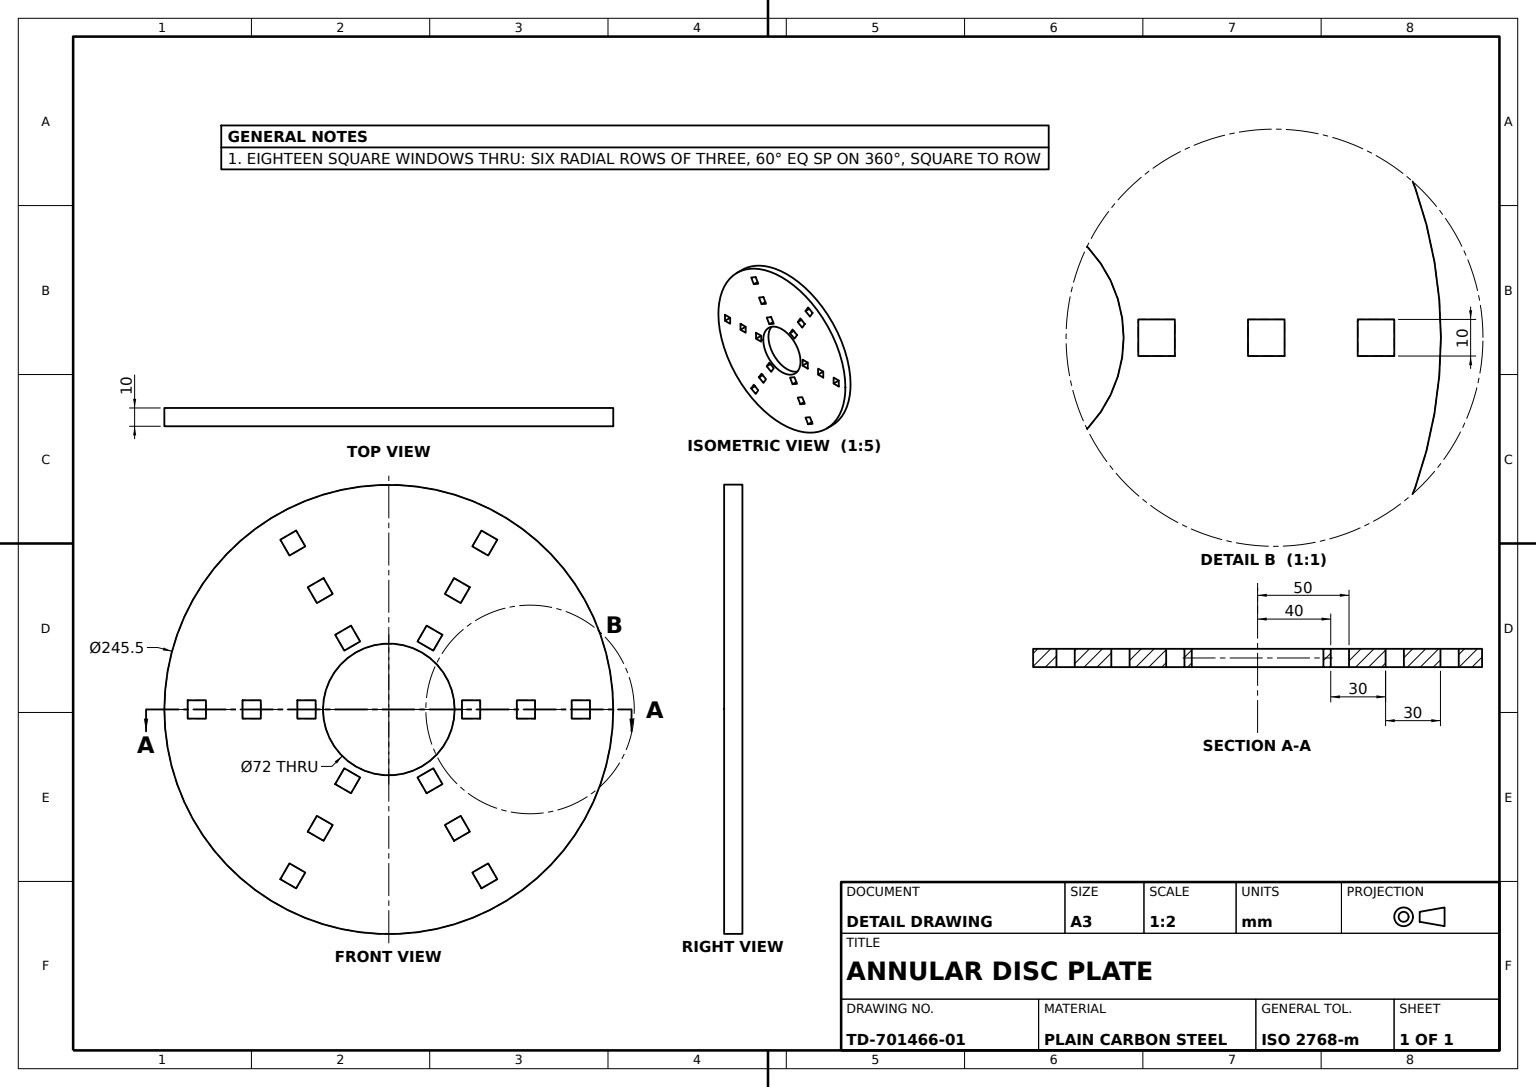
SolidWorks part; units mm, degrees
material "Plain Carbon Steel"
ref_plane "Front Plane" through (0, 0, 0) normal (0, 0, 1) x (1, 0, 0)
ref_plane "Top Plane" through (0, 0, 0) normal (0, 1, 0) x (1, 0, 0)
ref_plane "Right Plane" through (0, 0, 0) normal (1, 0, 0) x (0, 0, -1)
sketch "Plate Profile Ø245.5" plane through (0, 0, 0) normal (0, 0, 1) x (1, 0, 0)
  circle A0 centre (0, 0) radius 122.75
  dimension "D1" = 245.5
extrude "Plate Disc Ø245.5x10" add sketch "Plate Profile Ø245.5" along normal blind 10
sketch "Centre Bore Profile Ø72" plane through (0, 0, 10) normal (0, 0, 1) x (1, 0, 0)
  circle A0 centre (0, 0) radius 36
  dimension "D1" = 72
extrude "Centre Bore Ø72" cut sketch "Centre Bore Profile Ø72" against normal through all
sketch "Window Profile" plane through (0, 0, 10) normal (0, 0, 1) x (1, 0, 0)
  line L0 (0, 0) -> (0, 122.75) construction
  line L1 (0, 0) -> (0, -122.75) construction
  line L2 (0, 0) -> (40, 0)
  line L3 (0, 0) -> (-122.75, 0)
  line L4 (40, 0) -> (40, 5)
  line L5 (40, 0) -> (40, -5)
  line L6 (40, -5) -> (50, -5)
  line L7 (50, -5) -> (50, 5)
  line L8 (50, 5) -> (40, 5)
  line L9 (50, 0) -> (122.75, 0)
  circle A0 centre (0, 0) radius 122.75 construction
  circle A1 centre (0, 0) radius 36 construction
  dimension "D1" = 40
  dimension "D2" = 50
extrude "Window Cut" cut sketch "Window Profile" against normal through all contours L7 L8 L4 L5 L6
ref_plane "Plane1" through (0, 0, 0) normal (1, 0, 0) x (0, 0, -1)
pattern_circular "Inner Window Circular Pattern 6x" count 6 over 360 about axis through (0, 0, 0) along (0, 0, 1) of "Window Cut"
sketch "Radial Row Direction Line" plane through (0, 0, 10) normal (0, 0, 1) x (1, 0, 0)
  line L0 (0, 0) -> (122.75, 0) construction
  circle A0 centre (0, 0) radius 122.75 construction
pattern_linear "Window Radial Row 3x30" count 3 spacing 30 along (1, 0, 0) of "Window Cut"
pattern_circular "Window Row Circular Pattern 6x" count 6 over 360 about axis through (0, 0, 0) along (0, 0, 1) of "Window Radial Row 3x30"
